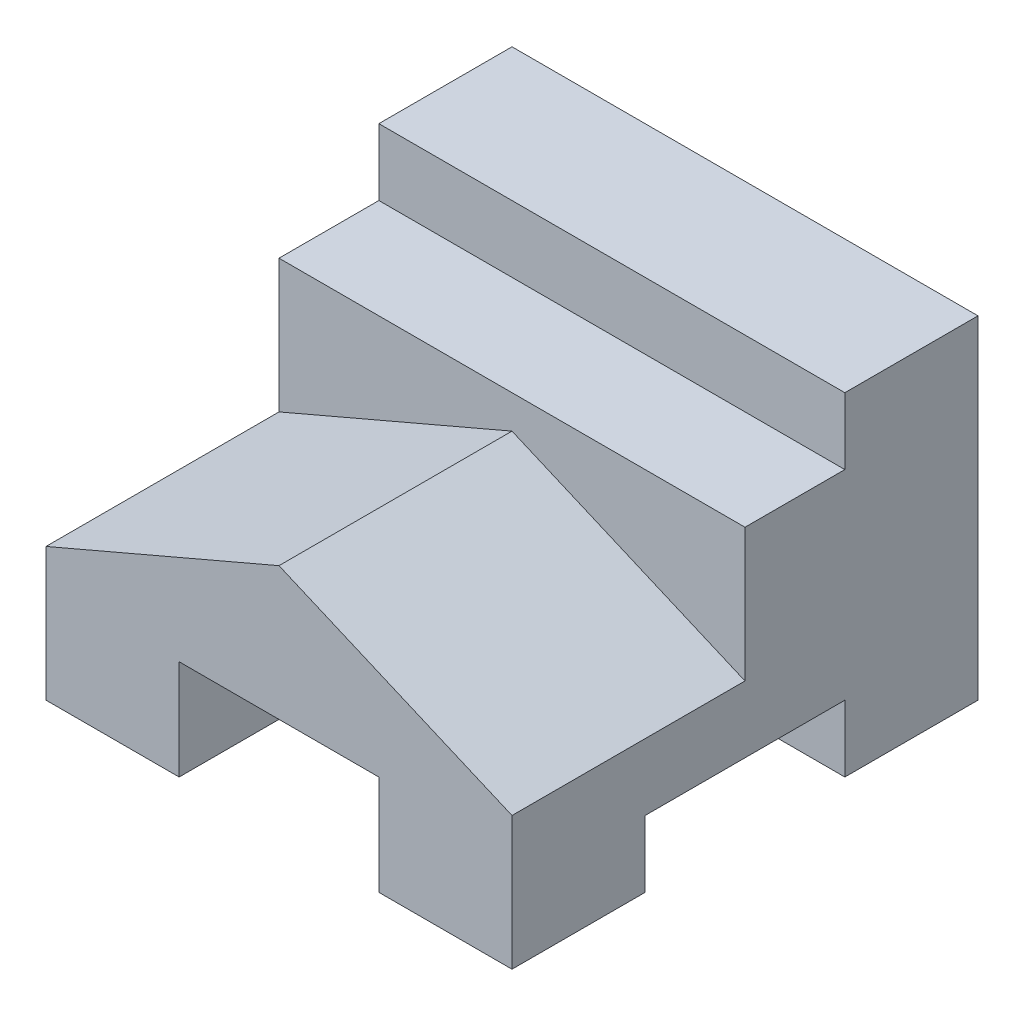
ISO-10303-21;
HEADER;
FILE_DESCRIPTION(('STEP AP214'),'2;1');
FILE_NAME('part.step','',(''),(''),'','','');
FILE_SCHEMA(('AUTOMOTIVE_DESIGN { 1 0 10303 214 1 1 1 1 }'));
ENDSEC;
DATA;
#1=APPLICATION_CONTEXT('core data for automotive mechanical design processes');
#2=APPLICATION_PROTOCOL_DEFINITION('international standard','automotive_design',2000,#1);
#3=PRODUCT_CONTEXT('',#1,'mechanical');
#4=PRODUCT('Part','Part','',(#3));
#5=PRODUCT_RELATED_PRODUCT_CATEGORY('part','',(#4));
#6=PRODUCT_DEFINITION_FORMATION('','',#4);
#7=PRODUCT_DEFINITION_CONTEXT('part definition',#1,'design');
#8=PRODUCT_DEFINITION('design','',#6,#7);
#9=PRODUCT_DEFINITION_SHAPE('','',#8);
#10=(LENGTH_UNIT() NAMED_UNIT(*) SI_UNIT(.MILLI.,.METRE.));
#11=(NAMED_UNIT(*) PLANE_ANGLE_UNIT() SI_UNIT($,.RADIAN.));
#12=(NAMED_UNIT(*) SI_UNIT($,.STERADIAN.) SOLID_ANGLE_UNIT());
#13=UNCERTAINTY_MEASURE_WITH_UNIT(LENGTH_MEASURE(1.E-05),#10,'distance_accuracy_value','');
#14=(GEOMETRIC_REPRESENTATION_CONTEXT(3) GLOBAL_UNCERTAINTY_ASSIGNED_CONTEXT((#13)) GLOBAL_UNIT_ASSIGNED_CONTEXT((#10,
#11,#12)) REPRESENTATION_CONTEXT('',''));
#15=CARTESIAN_POINT('',(0.,0.,0.));
#16=DIRECTION('',(0.,0.,1.));
#17=DIRECTION('',(1.,0.,0.));
#18=AXIS2_PLACEMENT_3D('',#15,#16,#17);
#19=CARTESIAN_POINT('',(70.,0.,50.));
#20=DIRECTION('',(0.,-1.,0.));
#21=DIRECTION('',(0.,0.,-1.));
#22=AXIS2_PLACEMENT_3D('',#19,#20,#21);
#23=PLANE('',#22);
#24=DIRECTION('',(0.,0.,1.));
#25=VECTOR('',#24,1.);
#26=CARTESIAN_POINT('',(20.,0.,35.));
#27=LINE('',#26,#25);
#28=CARTESIAN_POINT('',(20.,0.,50.));
#29=VERTEX_POINT('',#28);
#30=CARTESIAN_POINT('',(20.,0.,70.));
#31=VERTEX_POINT('',#30);
#32=EDGE_CURVE('E204',#29,#31,#27,.T.);
#33=ORIENTED_EDGE('',*,*,#32,.T.);
#34=DIRECTION('',(-1.,0.,0.));
#35=VECTOR('',#34,1.);
#36=CARTESIAN_POINT('',(70.,0.,70.));
#37=LINE('',#36,#35);
#38=CARTESIAN_POINT('',(0.,0.,70.));
#39=VERTEX_POINT('',#38);
#40=EDGE_CURVE('E275',#31,#39,#37,.T.);
#41=ORIENTED_EDGE('',*,*,#40,.T.);
#42=DIRECTION('',(0.,0.,1.));
#43=VECTOR('',#42,1.);
#44=CARTESIAN_POINT('',(0.,0.,50.));
#45=LINE('',#44,#43);
#46=CARTESIAN_POINT('',(0.,0.,50.));
#47=VERTEX_POINT('',#46);
#48=EDGE_CURVE('E246',#47,#39,#45,.T.);
#49=ORIENTED_EDGE('',*,*,#48,.F.);
#50=DIRECTION('',(-1.,0.,0.));
#51=VECTOR('',#50,1.);
#52=CARTESIAN_POINT('',(70.,0.,50.));
#53=LINE('',#52,#51);
#54=EDGE_CURVE('E277',#29,#47,#53,.T.);
#55=ORIENTED_EDGE('',*,*,#54,.F.);
#56=EDGE_LOOP('',(#33,#41,#49,#55));
#57=FACE_BOUND('',#56,.T.);
#58=ADVANCED_FACE('F44',(#57),#23,.T.);
#59=CARTESIAN_POINT('',(70.,10.,50.));
#60=DIRECTION('',(0.,0.,-1.));
#61=DIRECTION('',(-1.,0.,0.));
#62=AXIS2_PLACEMENT_3D('',#59,#60,#61);
#63=PLANE('',#62);
#64=DIRECTION('',(0.,1.,0.));
#65=VECTOR('',#64,1.);
#66=CARTESIAN_POINT('',(20.,10.,50.));
#67=LINE('',#66,#65);
#68=CARTESIAN_POINT('',(20.,10.,50.));
#69=VERTEX_POINT('',#68);
#70=EDGE_CURVE('E211',#29,#69,#67,.T.);
#71=ORIENTED_EDGE('',*,*,#70,.F.);
#72=ORIENTED_EDGE('',*,*,#54,.T.);
#73=DIRECTION('',(0.,-1.,0.));
#74=VECTOR('',#73,1.);
#75=CARTESIAN_POINT('',(0.,10.,50.));
#76=LINE('',#75,#74);
#77=CARTESIAN_POINT('',(0.,10.,50.));
#78=VERTEX_POINT('',#77);
#79=EDGE_CURVE('E249',#78,#47,#76,.T.);
#80=ORIENTED_EDGE('',*,*,#79,.F.);
#81=DIRECTION('',(-1.,0.,0.));
#82=VECTOR('',#81,1.);
#83=CARTESIAN_POINT('',(70.,10.,50.));
#84=LINE('',#83,#82);
#85=EDGE_CURVE('E278',#69,#78,#84,.T.);
#86=ORIENTED_EDGE('',*,*,#85,.F.);
#87=EDGE_LOOP('',(#71,#72,#80,#86));
#88=FACE_BOUND('',#87,.T.);
#89=ADVANCED_FACE('F380',(#88),#63,.T.);
#90=CARTESIAN_POINT('',(0.,0.,20.));
#91=DIRECTION('',(0.,0.,-1.));
#92=DIRECTION('',(-1.,0.,0.));
#93=AXIS2_PLACEMENT_3D('',#90,#91,#92);
#94=PLANE('',#93);
#95=DIRECTION('',(-1.,0.,0.));
#96=VECTOR('',#95,1.);
#97=CARTESIAN_POINT('',(70.,40.,20.));
#98=LINE('',#97,#96);
#99=CARTESIAN_POINT('',(70.,40.,20.));
#100=VERTEX_POINT('',#99);
#101=CARTESIAN_POINT('',(0.,40.,20.));
#102=VERTEX_POINT('',#101);
#103=EDGE_CURVE('E262',#100,#102,#98,.T.);
#104=ORIENTED_EDGE('',*,*,#103,.F.);
#105=DIRECTION('',(0.,1.,0.));
#106=VECTOR('',#105,1.);
#107=CARTESIAN_POINT('',(70.,50.,20.));
#108=LINE('',#107,#106);
#109=CARTESIAN_POINT('',(70.,50.,20.));
#110=VERTEX_POINT('',#109);
#111=EDGE_CURVE('E287',#100,#110,#108,.T.);
#112=ORIENTED_EDGE('',*,*,#111,.T.);
#113=DIRECTION('',(-1.,0.,0.));
#114=VECTOR('',#113,1.);
#115=CARTESIAN_POINT('',(0.,50.,20.));
#116=LINE('',#115,#114);
#117=CARTESIAN_POINT('',(0.,50.,20.));
#118=VERTEX_POINT('',#117);
#119=EDGE_CURVE('E295',#110,#118,#116,.T.);
#120=ORIENTED_EDGE('',*,*,#119,.T.);
#121=DIRECTION('',(0.,-1.,0.));
#122=VECTOR('',#121,1.);
#123=CARTESIAN_POINT('',(0.,0.,20.));
#124=LINE('',#123,#122);
#125=EDGE_CURVE('E285',#118,#102,#124,.T.);
#126=ORIENTED_EDGE('',*,*,#125,.T.);
#127=EDGE_LOOP('',(#104,#112,#120,#126));
#128=FACE_BOUND('',#127,.T.);
#129=ADVANCED_FACE('F349',(#128),#94,.F.);
#130=CARTESIAN_POINT('',(70.,0.,15.));
#131=DIRECTION('',(0.,1.,0.));
#132=DIRECTION('',(0.,0.,1.));
#133=AXIS2_PLACEMENT_3D('',#130,#131,#132);
#134=PLANE('',#133);
#135=DIRECTION('',(1.,0.,0.));
#136=VECTOR('',#135,1.);
#137=CARTESIAN_POINT('',(70.,0.,0.));
#138=LINE('',#137,#136);
#139=CARTESIAN_POINT('',(0.,0.,0.));
#140=VERTEX_POINT('',#139);
#141=CARTESIAN_POINT('',(70.,0.,0.));
#142=VERTEX_POINT('',#141);
#143=EDGE_CURVE('E293',#140,#142,#138,.T.);
#144=ORIENTED_EDGE('',*,*,#143,.T.);
#145=DIRECTION('',(0.,0.,-1.));
#146=VECTOR('',#145,1.);
#147=CARTESIAN_POINT('',(70.,0.,15.));
#148=LINE('',#147,#146);
#149=CARTESIAN_POINT('',(70.,0.,20.));
#150=VERTEX_POINT('',#149);
#151=EDGE_CURVE('E311',#150,#142,#148,.T.);
#152=ORIENTED_EDGE('',*,*,#151,.F.);
#153=DIRECTION('',(1.,0.,0.));
#154=VECTOR('',#153,1.);
#155=CARTESIAN_POINT('',(70.,0.,20.));
#156=LINE('',#155,#154);
#157=CARTESIAN_POINT('',(0.,0.,20.));
#158=VERTEX_POINT('',#157);
#159=EDGE_CURVE('E282',#158,#150,#156,.T.);
#160=ORIENTED_EDGE('',*,*,#159,.F.);
#161=DIRECTION('',(0.,0.,-1.));
#162=VECTOR('',#161,1.);
#163=CARTESIAN_POINT('',(0.,0.,15.));
#164=LINE('',#163,#162);
#165=EDGE_CURVE('E305',#158,#140,#164,.T.);
#166=ORIENTED_EDGE('',*,*,#165,.T.);
#167=EDGE_LOOP('',(#144,#152,#160,#166));
#168=FACE_BOUND('',#167,.T.);
#169=ADVANCED_FACE('F50',(#168),#134,.F.);
#170=CARTESIAN_POINT('',(70.,50.,15.));
#171=DIRECTION('',(-1.,0.,0.));
#172=DIRECTION('',(0.,0.,1.));
#173=AXIS2_PLACEMENT_3D('',#170,#171,#172);
#174=PLANE('',#173);
#175=DIRECTION('',(0.,1.,0.));
#176=VECTOR('',#175,1.);
#177=CARTESIAN_POINT('',(70.,50.,0.));
#178=LINE('',#177,#176);
#179=CARTESIAN_POINT('',(70.,50.,0.));
#180=VERTEX_POINT('',#179);
#181=EDGE_CURVE('E296',#142,#180,#178,.T.);
#182=ORIENTED_EDGE('',*,*,#181,.T.);
#183=DIRECTION('',(0.,0.,-1.));
#184=VECTOR('',#183,1.);
#185=CARTESIAN_POINT('',(70.,50.,15.));
#186=LINE('',#185,#184);
#187=EDGE_CURVE('E309',#110,#180,#186,.T.);
#188=ORIENTED_EDGE('',*,*,#187,.F.);
#189=ORIENTED_EDGE('',*,*,#111,.F.);
#190=DIRECTION('',(0.,0.,-1.));
#191=VECTOR('',#190,1.);
#192=CARTESIAN_POINT('',(70.,40.,20.));
#193=LINE('',#192,#191);
#194=CARTESIAN_POINT('',(70.,40.,35.));
#195=VERTEX_POINT('',#194);
#196=EDGE_CURVE('E241',#195,#100,#193,.T.);
#197=ORIENTED_EDGE('',*,*,#196,.F.);
#198=DIRECTION('',(0.,1.,0.));
#199=VECTOR('',#198,1.);
#200=CARTESIAN_POINT('',(70.,20.,35.));
#201=LINE('',#200,#199);
#202=CARTESIAN_POINT('',(70.,20.,35.));
#203=VERTEX_POINT('',#202);
#204=EDGE_CURVE('E238',#203,#195,#201,.T.);
#205=ORIENTED_EDGE('',*,*,#204,.F.);
#206=DIRECTION('',(0.,0.,-1.));
#207=VECTOR('',#206,1.);
#208=CARTESIAN_POINT('',(70.,20.,70.));
#209=LINE('',#208,#207);
#210=CARTESIAN_POINT('',(70.,20.,70.));
#211=VERTEX_POINT('',#210);
#212=EDGE_CURVE('E236',#211,#203,#209,.T.);
#213=ORIENTED_EDGE('',*,*,#212,.F.);
#214=DIRECTION('',(0.,1.,0.));
#215=VECTOR('',#214,1.);
#216=CARTESIAN_POINT('',(70.,0.,70.));
#217=LINE('',#216,#215);
#218=CARTESIAN_POINT('',(70.,0.,70.));
#219=VERTEX_POINT('',#218);
#220=EDGE_CURVE('E231',#219,#211,#217,.T.);
#221=ORIENTED_EDGE('',*,*,#220,.F.);
#222=DIRECTION('',(0.,0.,1.));
#223=VECTOR('',#222,1.);
#224=CARTESIAN_POINT('',(70.,0.,50.));
#225=LINE('',#224,#223);
#226=CARTESIAN_POINT('',(70.,0.,50.));
#227=VERTEX_POINT('',#226);
#228=EDGE_CURVE('E234',#227,#219,#225,.T.);
#229=ORIENTED_EDGE('',*,*,#228,.F.);
#230=DIRECTION('',(0.,-1.,0.));
#231=VECTOR('',#230,1.);
#232=CARTESIAN_POINT('',(70.,10.,50.));
#233=LINE('',#232,#231);
#234=CARTESIAN_POINT('',(70.,10.,50.));
#235=VERTEX_POINT('',#234);
#236=EDGE_CURVE('E226',#235,#227,#233,.T.);
#237=ORIENTED_EDGE('',*,*,#236,.F.);
#238=DIRECTION('',(0.,0.,1.));
#239=VECTOR('',#238,1.);
#240=CARTESIAN_POINT('',(70.,10.,20.));
#241=LINE('',#240,#239);
#242=CARTESIAN_POINT('',(70.,10.,20.));
#243=VERTEX_POINT('',#242);
#244=EDGE_CURVE('E223',#243,#235,#241,.T.);
#245=ORIENTED_EDGE('',*,*,#244,.F.);
#246=EDGE_CURVE('E290',#150,#243,#108,.T.);
#247=ORIENTED_EDGE('',*,*,#246,.F.);
#248=ORIENTED_EDGE('',*,*,#151,.T.);
#249=EDGE_LOOP('',(#182,#188,#189,#197,#205,#213,#221,#229,#237,#245,#247,#248));
#250=FACE_BOUND('',#249,.T.);
#251=ADVANCED_FACE('F326',(#250),#174,.F.);
#252=CARTESIAN_POINT('',(0.,50.,15.));
#253=DIRECTION('',(0.,-1.,0.));
#254=DIRECTION('',(0.,0.,-1.));
#255=AXIS2_PLACEMENT_3D('',#252,#253,#254);
#256=PLANE('',#255);
#257=DIRECTION('',(-1.,0.,0.));
#258=VECTOR('',#257,1.);
#259=CARTESIAN_POINT('',(0.,50.,0.));
#260=LINE('',#259,#258);
#261=CARTESIAN_POINT('',(0.,50.,0.));
#262=VERTEX_POINT('',#261);
#263=EDGE_CURVE('E297',#180,#262,#260,.T.);
#264=ORIENTED_EDGE('',*,*,#263,.T.);
#265=DIRECTION('',(0.,0.,-1.));
#266=VECTOR('',#265,1.);
#267=CARTESIAN_POINT('',(0.,50.,15.));
#268=LINE('',#267,#266);
#269=EDGE_CURVE('E307',#118,#262,#268,.T.);
#270=ORIENTED_EDGE('',*,*,#269,.F.);
#271=ORIENTED_EDGE('',*,*,#119,.F.);
#272=ORIENTED_EDGE('',*,*,#187,.T.);
#273=EDGE_LOOP('',(#264,#270,#271,#272));
#274=FACE_BOUND('',#273,.T.);
#275=ADVANCED_FACE('F343',(#274),#256,.F.);
#276=CARTESIAN_POINT('',(0.,0.,15.));
#277=DIRECTION('',(1.,0.,0.));
#278=DIRECTION('',(0.,0.,-1.));
#279=AXIS2_PLACEMENT_3D('',#276,#277,#278);
#280=PLANE('',#279);
#281=DIRECTION('',(0.,-1.,0.));
#282=VECTOR('',#281,1.);
#283=CARTESIAN_POINT('',(0.,0.,0.));
#284=LINE('',#283,#282);
#285=EDGE_CURVE('E304',#262,#140,#284,.T.);
#286=ORIENTED_EDGE('',*,*,#285,.T.);
#287=ORIENTED_EDGE('',*,*,#165,.F.);
#288=CARTESIAN_POINT('',(0.,10.,20.));
#289=VERTEX_POINT('',#288);
#290=EDGE_CURVE('E266',#289,#158,#124,.T.);
#291=ORIENTED_EDGE('',*,*,#290,.F.);
#292=DIRECTION('',(0.,0.,1.));
#293=VECTOR('',#292,1.);
#294=CARTESIAN_POINT('',(0.,10.,20.));
#295=LINE('',#294,#293);
#296=EDGE_CURVE('E69',#289,#78,#295,.T.);
#297=ORIENTED_EDGE('',*,*,#296,.T.);
#298=ORIENTED_EDGE('',*,*,#79,.T.);
#299=ORIENTED_EDGE('',*,*,#48,.T.);
#300=DIRECTION('',(0.,1.,0.));
#301=VECTOR('',#300,1.);
#302=CARTESIAN_POINT('',(0.,0.,70.));
#303=LINE('',#302,#301);
#304=CARTESIAN_POINT('',(0.,20.,70.));
#305=VERTEX_POINT('',#304);
#306=EDGE_CURVE('E251',#39,#305,#303,.T.);
#307=ORIENTED_EDGE('',*,*,#306,.T.);
#308=DIRECTION('',(0.,0.,-1.));
#309=VECTOR('',#308,1.);
#310=CARTESIAN_POINT('',(0.,20.,70.));
#311=LINE('',#310,#309);
#312=CARTESIAN_POINT('',(0.,20.,35.));
#313=VERTEX_POINT('',#312);
#314=EDGE_CURVE('E258',#305,#313,#311,.T.);
#315=ORIENTED_EDGE('',*,*,#314,.T.);
#316=DIRECTION('',(0.,1.,0.));
#317=VECTOR('',#316,1.);
#318=CARTESIAN_POINT('',(0.,20.,35.));
#319=LINE('',#318,#317);
#320=CARTESIAN_POINT('',(0.,40.,35.));
#321=VERTEX_POINT('',#320);
#322=EDGE_CURVE('E259',#313,#321,#319,.T.);
#323=ORIENTED_EDGE('',*,*,#322,.T.);
#324=DIRECTION('',(0.,0.,-1.));
#325=VECTOR('',#324,1.);
#326=CARTESIAN_POINT('',(0.,40.,20.));
#327=LINE('',#326,#325);
#328=EDGE_CURVE('E229',#321,#102,#327,.T.);
#329=ORIENTED_EDGE('',*,*,#328,.T.);
#330=ORIENTED_EDGE('',*,*,#125,.F.);
#331=ORIENTED_EDGE('',*,*,#269,.T.);
#332=EDGE_LOOP('',(#286,#287,#291,#297,#298,#299,#307,#315,#323,#329,#330,#331));
#333=FACE_BOUND('',#332,.T.);
#334=ADVANCED_FACE('F341',(#333),#280,.F.);
#335=CARTESIAN_POINT('',(0.,0.,0.));
#336=DIRECTION('',(0.,0.,-1.));
#337=DIRECTION('',(-1.,0.,0.));
#338=AXIS2_PLACEMENT_3D('',#335,#336,#337);
#339=PLANE('',#338);
#340=ORIENTED_EDGE('',*,*,#143,.F.);
#341=ORIENTED_EDGE('',*,*,#285,.F.);
#342=ORIENTED_EDGE('',*,*,#263,.F.);
#343=ORIENTED_EDGE('',*,*,#181,.F.);
#344=EDGE_LOOP('',(#340,#341,#342,#343));
#345=FACE_BOUND('',#344,.T.);
#346=ADVANCED_FACE('F342',(#345),#339,.T.);
#347=ORIENTED_EDGE('',*,*,#246,.T.);
#348=DIRECTION('',(-1.,0.,0.));
#349=VECTOR('',#348,1.);
#350=CARTESIAN_POINT('',(70.,10.,20.));
#351=LINE('',#350,#349);
#352=EDGE_CURVE('E242',#243,#289,#351,.T.);
#353=ORIENTED_EDGE('',*,*,#352,.T.);
#354=ORIENTED_EDGE('',*,*,#290,.T.);
#355=ORIENTED_EDGE('',*,*,#159,.T.);
#356=EDGE_LOOP('',(#347,#353,#354,#355));
#357=FACE_BOUND('',#356,.T.);
#358=ADVANCED_FACE('F328',(#357),#94,.F.);
#359=CARTESIAN_POINT('',(70.,40.,20.));
#360=DIRECTION('',(0.,1.,0.));
#361=DIRECTION('',(0.,0.,1.));
#362=AXIS2_PLACEMENT_3D('',#359,#360,#361);
#363=PLANE('',#362);
#364=ORIENTED_EDGE('',*,*,#328,.F.);
#365=DIRECTION('',(-1.,0.,0.));
#366=VECTOR('',#365,1.);
#367=CARTESIAN_POINT('',(70.,40.,35.));
#368=LINE('',#367,#366);
#369=EDGE_CURVE('E270',#195,#321,#368,.T.);
#370=ORIENTED_EDGE('',*,*,#369,.F.);
#371=ORIENTED_EDGE('',*,*,#196,.T.);
#372=ORIENTED_EDGE('',*,*,#103,.T.);
#373=EDGE_LOOP('',(#364,#370,#371,#372));
#374=FACE_BOUND('',#373,.T.);
#375=ADVANCED_FACE('F352',(#374),#363,.T.);
#376=CARTESIAN_POINT('',(70.,20.,35.));
#377=DIRECTION('',(0.,0.,1.));
#378=DIRECTION('',(0.,-1.,0.));
#379=AXIS2_PLACEMENT_3D('',#376,#377,#378);
#380=PLANE('',#379);
#381=DIRECTION('',(-0.919145030018058,0.393919298579168,0.));
#382=VECTOR('',#381,1.);
#383=CARTESIAN_POINT('',(70.,20.,35.));
#384=LINE('',#383,#382);
#385=CARTESIAN_POINT('',(35.,35.,35.));
#386=VERTEX_POINT('',#385);
#387=EDGE_CURVE('E212',#203,#386,#384,.T.);
#388=ORIENTED_EDGE('',*,*,#387,.F.);
#389=ORIENTED_EDGE('',*,*,#204,.T.);
#390=ORIENTED_EDGE('',*,*,#369,.T.);
#391=ORIENTED_EDGE('',*,*,#322,.F.);
#392=DIRECTION('',(-0.919145030018058,-0.393919298579168,0.));
#393=VECTOR('',#392,1.);
#394=CARTESIAN_POINT('',(35.,35.,35.));
#395=LINE('',#394,#393);
#396=EDGE_CURVE('E220',#386,#313,#395,.T.);
#397=ORIENTED_EDGE('',*,*,#396,.F.);
#398=EDGE_LOOP('',(#388,#389,#390,#391,#397));
#399=FACE_BOUND('',#398,.T.);
#400=ADVANCED_FACE('F360',(#399),#380,.T.);
#401=CARTESIAN_POINT('',(70.,0.,70.));
#402=DIRECTION('',(0.,0.,1.));
#403=DIRECTION('',(1.,0.,0.));
#404=AXIS2_PLACEMENT_3D('',#401,#402,#403);
#405=PLANE('',#404);
#406=DIRECTION('',(0.,-1.,0.));
#407=VECTOR('',#406,1.);
#408=CARTESIAN_POINT('',(20.,0.,70.));
#409=LINE('',#408,#407);
#410=CARTESIAN_POINT('',(20.,15.,70.));
#411=VERTEX_POINT('',#410);
#412=EDGE_CURVE('E181',#411,#31,#409,.T.);
#413=ORIENTED_EDGE('',*,*,#412,.F.);
#414=DIRECTION('',(-1.,0.,0.));
#415=VECTOR('',#414,1.);
#416=CARTESIAN_POINT('',(20.,15.,70.));
#417=LINE('',#416,#415);
#418=CARTESIAN_POINT('',(50.,15.,70.));
#419=VERTEX_POINT('',#418);
#420=EDGE_CURVE('E203',#419,#411,#417,.T.);
#421=ORIENTED_EDGE('',*,*,#420,.F.);
#422=DIRECTION('',(0.,1.,0.));
#423=VECTOR('',#422,1.);
#424=CARTESIAN_POINT('',(50.,15.,70.));
#425=LINE('',#424,#423);
#426=CARTESIAN_POINT('',(50.,0.,70.));
#427=VERTEX_POINT('',#426);
#428=EDGE_CURVE('E189',#427,#419,#425,.T.);
#429=ORIENTED_EDGE('',*,*,#428,.F.);
#430=EDGE_CURVE('E267',#219,#427,#37,.T.);
#431=ORIENTED_EDGE('',*,*,#430,.F.);
#432=ORIENTED_EDGE('',*,*,#220,.T.);
#433=DIRECTION('',(-0.919145030018058,0.393919298579168,0.));
#434=VECTOR('',#433,1.);
#435=CARTESIAN_POINT('',(70.,20.,70.));
#436=LINE('',#435,#434);
#437=CARTESIAN_POINT('',(35.,35.,70.));
#438=VERTEX_POINT('',#437);
#439=EDGE_CURVE('E213',#211,#438,#436,.T.);
#440=ORIENTED_EDGE('',*,*,#439,.T.);
#441=DIRECTION('',(-0.919145030018058,-0.393919298579168,0.));
#442=VECTOR('',#441,1.);
#443=CARTESIAN_POINT('',(35.,35.,70.));
#444=LINE('',#443,#442);
#445=EDGE_CURVE('E217',#438,#305,#444,.T.);
#446=ORIENTED_EDGE('',*,*,#445,.T.);
#447=ORIENTED_EDGE('',*,*,#306,.F.);
#448=ORIENTED_EDGE('',*,*,#40,.F.);
#449=EDGE_LOOP('',(#413,#421,#429,#431,#432,#440,#446,#447,#448));
#450=FACE_BOUND('',#449,.T.);
#451=ADVANCED_FACE('F370',(#450),#405,.T.);
#452=DIRECTION('',(0.,0.,1.));
#453=VECTOR('',#452,1.);
#454=CARTESIAN_POINT('',(50.,0.,35.));
#455=LINE('',#454,#453);
#456=CARTESIAN_POINT('',(50.,0.,50.));
#457=VERTEX_POINT('',#456);
#458=EDGE_CURVE('E195',#457,#427,#455,.T.);
#459=ORIENTED_EDGE('',*,*,#458,.F.);
#460=EDGE_CURVE('E272',#227,#457,#53,.T.);
#461=ORIENTED_EDGE('',*,*,#460,.F.);
#462=ORIENTED_EDGE('',*,*,#228,.T.);
#463=ORIENTED_EDGE('',*,*,#430,.T.);
#464=EDGE_LOOP('',(#459,#461,#462,#463));
#465=FACE_BOUND('',#464,.T.);
#466=ADVANCED_FACE('F369',(#465),#23,.T.);
#467=DIRECTION('',(0.,-1.,0.));
#468=VECTOR('',#467,1.);
#469=CARTESIAN_POINT('',(50.,10.,50.));
#470=LINE('',#469,#468);
#471=CARTESIAN_POINT('',(50.,10.,50.));
#472=VERTEX_POINT('',#471);
#473=EDGE_CURVE('E210',#472,#457,#470,.T.);
#474=ORIENTED_EDGE('',*,*,#473,.F.);
#475=EDGE_CURVE('E280',#235,#472,#84,.T.);
#476=ORIENTED_EDGE('',*,*,#475,.F.);
#477=ORIENTED_EDGE('',*,*,#236,.T.);
#478=ORIENTED_EDGE('',*,*,#460,.T.);
#479=EDGE_LOOP('',(#474,#476,#477,#478));
#480=FACE_BOUND('',#479,.T.);
#481=ADVANCED_FACE('F317',(#480),#63,.T.);
#482=CARTESIAN_POINT('',(70.,10.,20.));
#483=DIRECTION('',(0.,-1.,0.));
#484=DIRECTION('',(0.,0.,-1.));
#485=AXIS2_PLACEMENT_3D('',#482,#483,#484);
#486=PLANE('',#485);
#487=DIRECTION('',(0.,0.,-1.));
#488=VECTOR('',#487,1.);
#489=CARTESIAN_POINT('',(20.,10.,20.));
#490=LINE('',#489,#488);
#491=CARTESIAN_POINT('',(20.,10.,35.));
#492=VERTEX_POINT('',#491);
#493=EDGE_CURVE('E11',#69,#492,#490,.T.);
#494=ORIENTED_EDGE('',*,*,#493,.F.);
#495=ORIENTED_EDGE('',*,*,#85,.T.);
#496=ORIENTED_EDGE('',*,*,#296,.F.);
#497=ORIENTED_EDGE('',*,*,#352,.F.);
#498=ORIENTED_EDGE('',*,*,#244,.T.);
#499=ORIENTED_EDGE('',*,*,#475,.T.);
#500=DIRECTION('',(0.,0.,1.));
#501=VECTOR('',#500,1.);
#502=CARTESIAN_POINT('',(50.,10.,20.));
#503=LINE('',#502,#501);
#504=CARTESIAN_POINT('',(50.,10.,35.));
#505=VERTEX_POINT('',#504);
#506=EDGE_CURVE('E52',#505,#472,#503,.T.);
#507=ORIENTED_EDGE('',*,*,#506,.F.);
#508=DIRECTION('',(1.,0.,0.));
#509=VECTOR('',#508,1.);
#510=CARTESIAN_POINT('',(70.,10.,35.));
#511=LINE('',#510,#509);
#512=EDGE_CURVE('E176',#492,#505,#511,.T.);
#513=ORIENTED_EDGE('',*,*,#512,.F.);
#514=EDGE_LOOP('',(#494,#495,#496,#497,#498,#499,#507,#513));
#515=FACE_BOUND('',#514,.T.);
#516=ADVANCED_FACE('F325',(#515),#486,.T.);
#517=CARTESIAN_POINT('',(70.,20.,35.));
#518=DIRECTION('',(0.393919298579168,0.919145030018058,0.));
#519=DIRECTION('',(-0.919145030018058,0.393919298579168,0.));
#520=AXIS2_PLACEMENT_3D('',#517,#518,#519);
#521=PLANE('',#520);
#522=ORIENTED_EDGE('',*,*,#439,.F.);
#523=ORIENTED_EDGE('',*,*,#212,.T.);
#524=ORIENTED_EDGE('',*,*,#387,.T.);
#525=DIRECTION('',(0.,0.,1.));
#526=VECTOR('',#525,1.);
#527=CARTESIAN_POINT('',(35.,35.,35.));
#528=LINE('',#527,#526);
#529=EDGE_CURVE('E219',#386,#438,#528,.T.);
#530=ORIENTED_EDGE('',*,*,#529,.T.);
#531=EDGE_LOOP('',(#522,#523,#524,#530));
#532=FACE_BOUND('',#531,.T.);
#533=ADVANCED_FACE('F362',(#532),#521,.T.);
#534=CARTESIAN_POINT('',(35.,35.,35.));
#535=DIRECTION('',(-0.393919298579168,0.919145030018058,0.));
#536=DIRECTION('',(-0.919145030018058,-0.393919298579168,0.));
#537=AXIS2_PLACEMENT_3D('',#534,#535,#536);
#538=PLANE('',#537);
#539=ORIENTED_EDGE('',*,*,#445,.F.);
#540=ORIENTED_EDGE('',*,*,#529,.F.);
#541=ORIENTED_EDGE('',*,*,#396,.T.);
#542=ORIENTED_EDGE('',*,*,#314,.F.);
#543=EDGE_LOOP('',(#539,#540,#541,#542));
#544=FACE_BOUND('',#543,.T.);
#545=ADVANCED_FACE('F398',(#544),#538,.T.);
#546=CARTESIAN_POINT('',(20.,0.,35.));
#547=DIRECTION('',(-1.,0.,0.));
#548=DIRECTION('',(0.,0.,1.));
#549=AXIS2_PLACEMENT_3D('',#546,#547,#548);
#550=PLANE('',#549);
#551=ORIENTED_EDGE('',*,*,#70,.T.);
#552=ORIENTED_EDGE('',*,*,#493,.T.);
#553=DIRECTION('',(0.,-1.,0.));
#554=VECTOR('',#553,1.);
#555=CARTESIAN_POINT('',(20.,0.,35.));
#556=LINE('',#555,#554);
#557=CARTESIAN_POINT('',(20.,15.,35.));
#558=VERTEX_POINT('',#557);
#559=EDGE_CURVE('E58',#558,#492,#556,.T.);
#560=ORIENTED_EDGE('',*,*,#559,.F.);
#561=DIRECTION('',(0.,0.,1.));
#562=VECTOR('',#561,1.);
#563=CARTESIAN_POINT('',(20.,15.,35.));
#564=LINE('',#563,#562);
#565=EDGE_CURVE('E192',#558,#411,#564,.T.);
#566=ORIENTED_EDGE('',*,*,#565,.T.);
#567=ORIENTED_EDGE('',*,*,#412,.T.);
#568=ORIENTED_EDGE('',*,*,#32,.F.);
#569=EDGE_LOOP('',(#551,#552,#560,#566,#567,#568));
#570=FACE_BOUND('',#569,.T.);
#571=ADVANCED_FACE('F394',(#570),#550,.F.);
#572=CARTESIAN_POINT('',(20.,15.,35.));
#573=DIRECTION('',(0.,1.,0.));
#574=DIRECTION('',(0.,0.,1.));
#575=AXIS2_PLACEMENT_3D('',#572,#573,#574);
#576=PLANE('',#575);
#577=ORIENTED_EDGE('',*,*,#420,.T.);
#578=ORIENTED_EDGE('',*,*,#565,.F.);
#579=DIRECTION('',(-1.,0.,0.));
#580=VECTOR('',#579,1.);
#581=CARTESIAN_POINT('',(20.,15.,35.));
#582=LINE('',#581,#580);
#583=CARTESIAN_POINT('',(50.,15.,35.));
#584=VERTEX_POINT('',#583);
#585=EDGE_CURVE('E177',#584,#558,#582,.T.);
#586=ORIENTED_EDGE('',*,*,#585,.F.);
#587=DIRECTION('',(0.,0.,1.));
#588=VECTOR('',#587,1.);
#589=CARTESIAN_POINT('',(50.,15.,35.));
#590=LINE('',#589,#588);
#591=EDGE_CURVE('E188',#584,#419,#590,.T.);
#592=ORIENTED_EDGE('',*,*,#591,.T.);
#593=EDGE_LOOP('',(#577,#578,#586,#592));
#594=FACE_BOUND('',#593,.T.);
#595=ADVANCED_FACE('F198',(#594),#576,.F.);
#596=CARTESIAN_POINT('',(50.,15.,35.));
#597=DIRECTION('',(1.,0.,0.));
#598=DIRECTION('',(0.,0.,-1.));
#599=AXIS2_PLACEMENT_3D('',#596,#597,#598);
#600=PLANE('',#599);
#601=ORIENTED_EDGE('',*,*,#473,.T.);
#602=ORIENTED_EDGE('',*,*,#458,.T.);
#603=ORIENTED_EDGE('',*,*,#428,.T.);
#604=ORIENTED_EDGE('',*,*,#591,.F.);
#605=DIRECTION('',(0.,1.,0.));
#606=VECTOR('',#605,1.);
#607=CARTESIAN_POINT('',(50.,15.,35.));
#608=LINE('',#607,#606);
#609=EDGE_CURVE('E174',#505,#584,#608,.T.);
#610=ORIENTED_EDGE('',*,*,#609,.F.);
#611=ORIENTED_EDGE('',*,*,#506,.T.);
#612=EDGE_LOOP('',(#601,#602,#603,#604,#610,#611));
#613=FACE_BOUND('',#612,.T.);
#614=ADVANCED_FACE('F190',(#613),#600,.F.);
#615=CARTESIAN_POINT('',(0.,0.,35.));
#616=DIRECTION('',(0.,0.,-1.));
#617=DIRECTION('',(-1.,0.,0.));
#618=AXIS2_PLACEMENT_3D('',#615,#616,#617);
#619=PLANE('',#618);
#620=ORIENTED_EDGE('',*,*,#512,.T.);
#621=ORIENTED_EDGE('',*,*,#609,.T.);
#622=ORIENTED_EDGE('',*,*,#585,.T.);
#623=ORIENTED_EDGE('',*,*,#559,.T.);
#624=EDGE_LOOP('',(#620,#621,#622,#623));
#625=FACE_BOUND('',#624,.T.);
#626=ADVANCED_FACE('F178',(#625),#619,.F.);
#627=CLOSED_SHELL('',(#58,#89,#129,#169,#251,#275,#334,#346,#358,#375,#400,#451,#466,#481,#516,
#533,#545,#571,#595,#614,#626));
#628=MANIFOLD_SOLID_BREP('B2',#627);
#629=ADVANCED_BREP_SHAPE_REPRESENTATION('',(#18,#628),#14);
#630=SHAPE_DEFINITION_REPRESENTATION(#9,#629);
ENDSEC;
END-ISO-10303-21;
